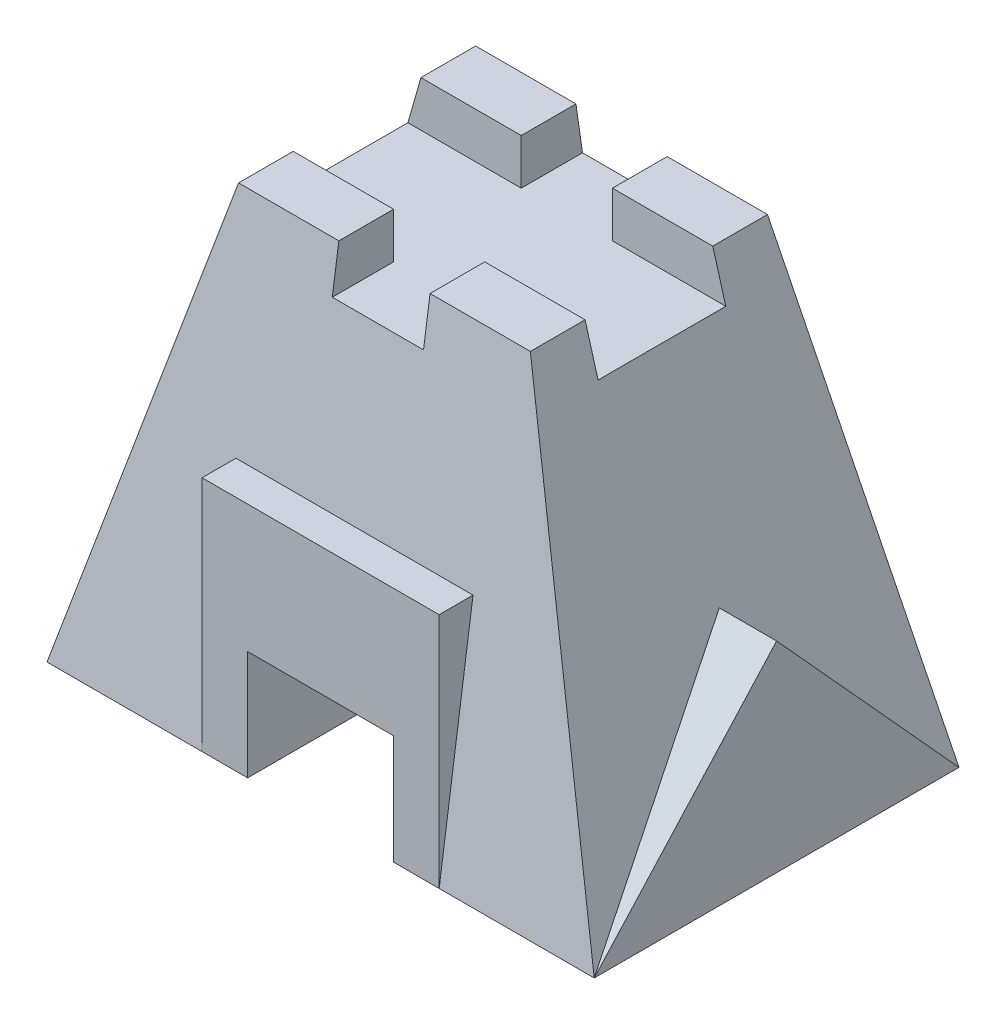
ISO-10303-21;
HEADER;
FILE_DESCRIPTION(('STEP AP214'),'2;1');
FILE_NAME('part.step','',(''),(''),'','','');
FILE_SCHEMA(('AUTOMOTIVE_DESIGN { 1 0 10303 214 1 1 1 1 }'));
ENDSEC;
DATA;
#1=APPLICATION_CONTEXT('core data for automotive mechanical design processes');
#2=APPLICATION_PROTOCOL_DEFINITION('international standard','automotive_design',2000,#1);
#3=PRODUCT_CONTEXT('',#1,'mechanical');
#4=PRODUCT('Part','Part','',(#3));
#5=PRODUCT_RELATED_PRODUCT_CATEGORY('part','',(#4));
#6=PRODUCT_DEFINITION_FORMATION('','',#4);
#7=PRODUCT_DEFINITION_CONTEXT('part definition',#1,'design');
#8=PRODUCT_DEFINITION('design','',#6,#7);
#9=PRODUCT_DEFINITION_SHAPE('','',#8);
#10=(LENGTH_UNIT() NAMED_UNIT(*) SI_UNIT(.MILLI.,.METRE.));
#11=(NAMED_UNIT(*) PLANE_ANGLE_UNIT() SI_UNIT($,.RADIAN.));
#12=(NAMED_UNIT(*) SI_UNIT($,.STERADIAN.) SOLID_ANGLE_UNIT());
#13=UNCERTAINTY_MEASURE_WITH_UNIT(LENGTH_MEASURE(1.E-05),#10,'distance_accuracy_value','');
#14=(GEOMETRIC_REPRESENTATION_CONTEXT(3) GLOBAL_UNCERTAINTY_ASSIGNED_CONTEXT((#13)) GLOBAL_UNIT_ASSIGNED_CONTEXT((#10,
#11,#12)) REPRESENTATION_CONTEXT('',''));
#15=CARTESIAN_POINT('',(0.,0.,0.));
#16=DIRECTION('',(0.,0.,1.));
#17=DIRECTION('',(1.,0.,0.));
#18=AXIS2_PLACEMENT_3D('',#15,#16,#17);
#19=CARTESIAN_POINT('',(0.,245.,0.));
#20=DIRECTION('',(0.,-1.,0.));
#21=DIRECTION('',(0.,0.,-1.));
#22=AXIS2_PLACEMENT_3D('',#19,#20,#21);
#23=PLANE('',#22);
#24=DIRECTION('',(-1.,0.,0.));
#25=VECTOR('',#24,1.);
#26=CARTESIAN_POINT('',(-80.,245.,-65.));
#27=LINE('',#26,#25);
#28=CARTESIAN_POINT('',(80.,245.,-65.));
#29=VERTEX_POINT('',#28);
#30=CARTESIAN_POINT('',(25.,245.,-65.));
#31=VERTEX_POINT('',#30);
#32=EDGE_CURVE('E51',#29,#31,#27,.T.);
#33=ORIENTED_EDGE('',*,*,#32,.T.);
#34=DIRECTION('',(0.,0.,-1.));
#35=VECTOR('',#34,1.);
#36=CARTESIAN_POINT('',(25.,245.,-74.6053871623696));
#37=LINE('',#36,#35);
#38=CARTESIAN_POINT('',(25.,245.,-35.));
#39=VERTEX_POINT('',#38);
#40=EDGE_CURVE('E244',#39,#31,#37,.T.);
#41=ORIENTED_EDGE('',*,*,#40,.F.);
#42=DIRECTION('',(1.,0.,0.));
#43=VECTOR('',#42,1.);
#44=CARTESIAN_POINT('',(0.,245.,-35.));
#45=LINE('',#44,#43);
#46=CARTESIAN_POINT('',(80.,245.,-35.));
#47=VERTEX_POINT('',#46);
#48=EDGE_CURVE('E60',#39,#47,#45,.T.);
#49=ORIENTED_EDGE('',*,*,#48,.T.);
#50=DIRECTION('',(0.,0.,-1.));
#51=VECTOR('',#50,1.);
#52=CARTESIAN_POINT('',(80.,245.,65.));
#53=LINE('',#52,#51);
#54=EDGE_CURVE('E428',#47,#29,#53,.T.);
#55=ORIENTED_EDGE('',*,*,#54,.T.);
#56=EDGE_LOOP('',(#33,#41,#49,#55));
#57=FACE_BOUND('',#56,.T.);
#58=ADVANCED_FACE('F50',(#57),#23,.F.);
#59=CARTESIAN_POINT('',(80.,245.,65.));
#60=VERTEX_POINT('',#59);
#61=CARTESIAN_POINT('',(80.,245.,35.));
#62=VERTEX_POINT('',#61);
#63=EDGE_CURVE('E536',#60,#62,#53,.T.);
#64=ORIENTED_EDGE('',*,*,#63,.T.);
#65=DIRECTION('',(1.,0.,0.));
#66=VECTOR('',#65,1.);
#67=CARTESIAN_POINT('',(80.,245.,35.));
#68=LINE('',#67,#66);
#69=CARTESIAN_POINT('',(25.,245.,35.));
#70=VERTEX_POINT('',#69);
#71=EDGE_CURVE('E292',#70,#62,#68,.T.);
#72=ORIENTED_EDGE('',*,*,#71,.F.);
#73=DIRECTION('',(0.,0.,1.));
#74=VECTOR('',#73,1.);
#75=CARTESIAN_POINT('',(25.,245.,0.));
#76=LINE('',#75,#74);
#77=CARTESIAN_POINT('',(25.,245.,65.));
#78=VERTEX_POINT('',#77);
#79=EDGE_CURVE('E552',#70,#78,#76,.T.);
#80=ORIENTED_EDGE('',*,*,#79,.T.);
#81=DIRECTION('',(1.,0.,0.));
#82=VECTOR('',#81,1.);
#83=CARTESIAN_POINT('',(-80.,245.,65.));
#84=LINE('',#83,#82);
#85=EDGE_CURVE('E531',#78,#60,#84,.T.);
#86=ORIENTED_EDGE('',*,*,#85,.T.);
#87=EDGE_LOOP('',(#64,#72,#80,#86));
#88=FACE_BOUND('',#87,.T.);
#89=ADVANCED_FACE('F750',(#88),#23,.F.);
#90=CARTESIAN_POINT('',(-80.,245.,65.));
#91=VERTEX_POINT('',#90);
#92=CARTESIAN_POINT('',(-25.,245.,65.));
#93=VERTEX_POINT('',#92);
#94=EDGE_CURVE('E529',#91,#93,#84,.T.);
#95=ORIENTED_EDGE('',*,*,#94,.T.);
#96=DIRECTION('',(0.,0.,1.));
#97=VECTOR('',#96,1.);
#98=CARTESIAN_POINT('',(-25.,245.,65.));
#99=LINE('',#98,#97);
#100=CARTESIAN_POINT('',(-25.,245.,35.));
#101=VERTEX_POINT('',#100);
#102=EDGE_CURVE('E276',#101,#93,#99,.T.);
#103=ORIENTED_EDGE('',*,*,#102,.F.);
#104=DIRECTION('',(-1.,0.,0.));
#105=VECTOR('',#104,1.);
#106=CARTESIAN_POINT('',(0.,245.,35.));
#107=LINE('',#106,#105);
#108=CARTESIAN_POINT('',(-80.,245.,35.));
#109=VERTEX_POINT('',#108);
#110=EDGE_CURVE('E557',#101,#109,#107,.T.);
#111=ORIENTED_EDGE('',*,*,#110,.T.);
#112=DIRECTION('',(0.,0.,1.));
#113=VECTOR('',#112,1.);
#114=CARTESIAN_POINT('',(-80.,245.,65.));
#115=LINE('',#114,#113);
#116=EDGE_CURVE('E545',#109,#91,#115,.T.);
#117=ORIENTED_EDGE('',*,*,#116,.T.);
#118=EDGE_LOOP('',(#95,#103,#111,#117));
#119=FACE_BOUND('',#118,.T.);
#120=ADVANCED_FACE('F451',(#119),#23,.F.);
#121=CARTESIAN_POINT('',(0.,0.,0.));
#122=DIRECTION('',(0.,-1.,0.));
#123=DIRECTION('',(0.,0.,-1.));
#124=AXIS2_PLACEMENT_3D('',#121,#122,#123);
#125=PLANE('',#124);
#126=DIRECTION('',(0.,0.,1.));
#127=VECTOR('',#126,1.);
#128=CARTESIAN_POINT('',(-40.,0.,-100.0001));
#129=LINE('',#128,#127);
#130=CARTESIAN_POINT('',(-40.,0.,-100.));
#131=VERTEX_POINT('',#130);
#132=CARTESIAN_POINT('',(-40.,0.,100.));
#133=VERTEX_POINT('',#132);
#134=EDGE_CURVE('E322',#131,#133,#129,.T.);
#135=ORIENTED_EDGE('',*,*,#134,.T.);
#136=DIRECTION('',(1.,0.,0.));
#137=VECTOR('',#136,1.);
#138=CARTESIAN_POINT('',(-65.,0.,100.));
#139=LINE('',#138,#137);
#140=CARTESIAN_POINT('',(-65.,0.,100.));
#141=VERTEX_POINT('',#140);
#142=EDGE_CURVE('E411',#141,#133,#139,.T.);
#143=ORIENTED_EDGE('',*,*,#142,.F.);
#144=DIRECTION('',(1.,0.,0.));
#145=VECTOR('',#144,1.);
#146=CARTESIAN_POINT('',(-150.,0.,100.));
#147=LINE('',#146,#145);
#148=CARTESIAN_POINT('',(-150.,0.,100.));
#149=VERTEX_POINT('',#148);
#150=EDGE_CURVE('E665',#149,#141,#147,.T.);
#151=ORIENTED_EDGE('',*,*,#150,.F.);
#152=DIRECTION('',(0.,0.,1.));
#153=VECTOR('',#152,1.);
#154=CARTESIAN_POINT('',(-150.,0.,100.));
#155=LINE('',#154,#153);
#156=CARTESIAN_POINT('',(-150.,0.,-100.));
#157=VERTEX_POINT('',#156);
#158=EDGE_CURVE('E654',#157,#149,#155,.T.);
#159=ORIENTED_EDGE('',*,*,#158,.F.);
#160=DIRECTION('',(-1.,0.,0.));
#161=VECTOR('',#160,1.);
#162=CARTESIAN_POINT('',(-150.,0.,-100.));
#163=LINE('',#162,#161);
#164=CARTESIAN_POINT('',(-65.,0.,-100.));
#165=VERTEX_POINT('',#164);
#166=EDGE_CURVE('E650',#165,#157,#163,.T.);
#167=ORIENTED_EDGE('',*,*,#166,.F.);
#168=DIRECTION('',(1.,0.,0.));
#169=VECTOR('',#168,1.);
#170=CARTESIAN_POINT('',(-65.,0.,-100.));
#171=LINE('',#170,#169);
#172=EDGE_CURVE('E406',#165,#131,#171,.T.);
#173=ORIENTED_EDGE('',*,*,#172,.T.);
#174=EDGE_LOOP('',(#135,#143,#151,#159,#167,#173));
#175=FACE_BOUND('',#174,.T.);
#176=ADVANCED_FACE('F709',(#175),#125,.T.);
#177=CARTESIAN_POINT('',(-138.679245283019,39.622641509434,0.));
#178=DIRECTION('',(-0.961523947640823,0.274721127897378,0.));
#179=DIRECTION('',(-0.274721127897378,-0.961523947640823,0.));
#180=AXIS2_PLACEMENT_3D('',#177,#178,#179);
#181=PLANE('',#180);
#182=DIRECTION('',(0.274721127897378,0.961523947640823,0.));
#183=VECTOR('',#182,1.);
#184=CARTESIAN_POINT('',(-138.679245283019,39.622641509434,35.));
#185=LINE('',#184,#183);
#186=CARTESIAN_POINT('',(-87.1428571428572,220.,35.));
#187=VERTEX_POINT('',#186);
#188=EDGE_CURVE('E285',#187,#109,#185,.T.);
#189=ORIENTED_EDGE('',*,*,#188,.F.);
#190=DIRECTION('',(0.,0.,1.));
#191=VECTOR('',#190,1.);
#192=CARTESIAN_POINT('',(-87.1428571428572,220.,0.));
#193=LINE('',#192,#191);
#194=CARTESIAN_POINT('',(-87.1428571428572,220.,-35.));
#195=VERTEX_POINT('',#194);
#196=EDGE_CURVE('E325',#195,#187,#193,.T.);
#197=ORIENTED_EDGE('',*,*,#196,.F.);
#198=DIRECTION('',(-0.274721127897378,-0.961523947640823,0.));
#199=VECTOR('',#198,1.);
#200=CARTESIAN_POINT('',(-138.679245283019,39.622641509434,-35.));
#201=LINE('',#200,#199);
#202=CARTESIAN_POINT('',(-80.,245.,-35.));
#203=VERTEX_POINT('',#202);
#204=EDGE_CURVE('E254',#203,#195,#201,.T.);
#205=ORIENTED_EDGE('',*,*,#204,.F.);
#206=CARTESIAN_POINT('',(-80.,245.,-65.));
#207=VERTEX_POINT('',#206);
#208=EDGE_CURVE('E532',#207,#203,#115,.T.);
#209=ORIENTED_EDGE('',*,*,#208,.F.);
#210=DIRECTION('',(-0.272165526975909,-0.95257934441568,-0.136082763487954));
#211=VECTOR('',#210,1.);
#212=CARTESIAN_POINT('',(-80.,245.,-65.));
#213=LINE('',#212,#211);
#214=EDGE_CURVE('E581',#207,#157,#213,.T.);
#215=ORIENTED_EDGE('',*,*,#214,.T.);
#216=DIRECTION('',(0.20683964668639,0.723938763402365,0.658126148547605));
#217=VECTOR('',#216,1.);
#218=CARTESIAN_POINT('',(-129.969946079731,70.1051887209405,-36.2680102536904));
#219=LINE('',#218,#217);
#220=CARTESIAN_POINT('',(-118.571428571429,110.,0.));
#221=VERTEX_POINT('',#220);
#222=EDGE_CURVE('E367',#157,#221,#219,.T.);
#223=ORIENTED_EDGE('',*,*,#222,.T.);
#224=DIRECTION('',(-0.20683964668639,-0.723938763402365,0.658126148547605));
#225=VECTOR('',#224,1.);
#226=CARTESIAN_POINT('',(-129.969946079731,70.1051887209405,36.2680102536904));
#227=LINE('',#226,#225);
#228=EDGE_CURVE('E355',#221,#149,#227,.T.);
#229=ORIENTED_EDGE('',*,*,#228,.T.);
#230=DIRECTION('',(-0.272165526975909,-0.95257934441568,0.136082763487954));
#231=VECTOR('',#230,1.);
#232=CARTESIAN_POINT('',(-80.,245.,65.));
#233=LINE('',#232,#231);
#234=EDGE_CURVE('E573',#91,#149,#233,.T.);
#235=ORIENTED_EDGE('',*,*,#234,.F.);
#236=ORIENTED_EDGE('',*,*,#116,.F.);
#237=EDGE_LOOP('',(#189,#197,#205,#209,#215,#223,#229,#235,#236));
#238=FACE_BOUND('',#237,.T.);
#239=ADVANCED_FACE('F460',(#238),#181,.T.);
#240=CARTESIAN_POINT('',(138.679245283019,39.6226415094339,0.));
#241=DIRECTION('',(0.961523947640823,0.274721127897378,0.));
#242=DIRECTION('',(-0.274721127897378,0.961523947640823,0.));
#243=AXIS2_PLACEMENT_3D('',#240,#241,#242);
#244=PLANE('',#243);
#245=DIRECTION('',(-0.274721127897378,0.961523947640823,0.));
#246=VECTOR('',#245,1.);
#247=CARTESIAN_POINT('',(138.679245283019,39.6226415094339,-35.));
#248=LINE('',#247,#246);
#249=CARTESIAN_POINT('',(87.1428571428571,220.,-35.));
#250=VERTEX_POINT('',#249);
#251=EDGE_CURVE('E316',#250,#47,#248,.T.);
#252=ORIENTED_EDGE('',*,*,#251,.F.);
#253=DIRECTION('',(0.,0.,-1.));
#254=VECTOR('',#253,1.);
#255=CARTESIAN_POINT('',(87.1428571428571,220.,0.));
#256=LINE('',#255,#254);
#257=CARTESIAN_POINT('',(87.1428571428571,220.,35.));
#258=VERTEX_POINT('',#257);
#259=EDGE_CURVE('E319',#258,#250,#256,.T.);
#260=ORIENTED_EDGE('',*,*,#259,.F.);
#261=DIRECTION('',(0.274721127897378,-0.961523947640823,0.));
#262=VECTOR('',#261,1.);
#263=CARTESIAN_POINT('',(138.679245283019,39.6226415094339,35.));
#264=LINE('',#263,#262);
#265=EDGE_CURVE('E299',#62,#258,#264,.T.);
#266=ORIENTED_EDGE('',*,*,#265,.F.);
#267=ORIENTED_EDGE('',*,*,#63,.F.);
#268=DIRECTION('',(0.272165526975909,-0.95257934441568,0.136082763487954));
#269=VECTOR('',#268,1.);
#270=CARTESIAN_POINT('',(80.,245.,65.));
#271=LINE('',#270,#269);
#272=CARTESIAN_POINT('',(150.,0.,100.));
#273=VERTEX_POINT('',#272);
#274=EDGE_CURVE('E588',#60,#273,#271,.T.);
#275=ORIENTED_EDGE('',*,*,#274,.T.);
#276=DIRECTION('',(-0.20683964668639,0.723938763402365,-0.658126148547605));
#277=VECTOR('',#276,1.);
#278=CARTESIAN_POINT('',(129.969946079731,70.1051887209405,36.2680102536904));
#279=LINE('',#278,#277);
#280=CARTESIAN_POINT('',(118.571428571429,110.,0.));
#281=VERTEX_POINT('',#280);
#282=EDGE_CURVE('E341',#273,#281,#279,.T.);
#283=ORIENTED_EDGE('',*,*,#282,.T.);
#284=DIRECTION('',(0.20683964668639,-0.723938763402365,-0.658126148547605));
#285=VECTOR('',#284,1.);
#286=CARTESIAN_POINT('',(129.969946079731,70.1051887209405,-36.2680102536904));
#287=LINE('',#286,#285);
#288=CARTESIAN_POINT('',(150.,0.,-100.));
#289=VERTEX_POINT('',#288);
#290=EDGE_CURVE('E365',#281,#289,#287,.T.);
#291=ORIENTED_EDGE('',*,*,#290,.T.);
#292=DIRECTION('',(0.272165526975909,-0.95257934441568,-0.136082763487954));
#293=VECTOR('',#292,1.);
#294=CARTESIAN_POINT('',(80.,245.,-65.));
#295=LINE('',#294,#293);
#296=EDGE_CURVE('E500',#29,#289,#295,.T.);
#297=ORIENTED_EDGE('',*,*,#296,.F.);
#298=ORIENTED_EDGE('',*,*,#54,.F.);
#299=EDGE_LOOP('',(#252,#260,#266,#267,#275,#283,#291,#297,#298));
#300=FACE_BOUND('',#299,.T.);
#301=ADVANCED_FACE('F508',(#300),#244,.T.);
#302=CARTESIAN_POINT('',(0.,14.,98.));
#303=DIRECTION('',(0.,0.141421356237309,0.989949493661167));
#304=DIRECTION('',(0.,-0.989949493661167,0.141421356237309));
#305=AXIS2_PLACEMENT_3D('',#302,#303,#304);
#306=PLANE('',#305);
#307=DIRECTION('',(0.,0.989949493661167,-0.141421356237309));
#308=VECTOR('',#307,1.);
#309=CARTESIAN_POINT('',(25.0000000000001,14.,98.));
#310=LINE('',#309,#308);
#311=CARTESIAN_POINT('',(25.,220.,68.5714285714286));
#312=VERTEX_POINT('',#311);
#313=EDGE_CURVE('E291',#312,#78,#310,.T.);
#314=ORIENTED_EDGE('',*,*,#313,.F.);
#315=DIRECTION('',(1.,0.,0.));
#316=VECTOR('',#315,1.);
#317=CARTESIAN_POINT('',(0.,220.,68.5714285714286));
#318=LINE('',#317,#316);
#319=CARTESIAN_POINT('',(-25.,220.,68.5714285714286));
#320=VERTEX_POINT('',#319);
#321=EDGE_CURVE('E312',#320,#312,#318,.T.);
#322=ORIENTED_EDGE('',*,*,#321,.F.);
#323=DIRECTION('',(0.,-0.989949493661167,0.141421356237309));
#324=VECTOR('',#323,1.);
#325=CARTESIAN_POINT('',(-25.,14.,98.));
#326=LINE('',#325,#324);
#327=EDGE_CURVE('E290',#93,#320,#326,.T.);
#328=ORIENTED_EDGE('',*,*,#327,.F.);
#329=ORIENTED_EDGE('',*,*,#94,.F.);
#330=ORIENTED_EDGE('',*,*,#234,.T.);
#331=ORIENTED_EDGE('',*,*,#150,.T.);
#332=DIRECTION('',(0.,0.989949493661167,-0.141421356237309));
#333=VECTOR('',#332,1.);
#334=CARTESIAN_POINT('',(-65.,14.,98.));
#335=LINE('',#334,#333);
#336=CARTESIAN_POINT('',(-65.,130.,81.4285714285714));
#337=VERTEX_POINT('',#336);
#338=EDGE_CURVE('E393',#141,#337,#335,.T.);
#339=ORIENTED_EDGE('',*,*,#338,.T.);
#340=DIRECTION('',(1.,0.,0.));
#341=VECTOR('',#340,1.);
#342=CARTESIAN_POINT('',(0.,130.,81.4285714285714));
#343=LINE('',#342,#341);
#344=CARTESIAN_POINT('',(65.,130.,81.4285714285714));
#345=VERTEX_POINT('',#344);
#346=EDGE_CURVE('E399',#337,#345,#343,.T.);
#347=ORIENTED_EDGE('',*,*,#346,.T.);
#348=DIRECTION('',(0.,-0.989949493661167,0.141421356237309));
#349=VECTOR('',#348,1.);
#350=CARTESIAN_POINT('',(65.,14.,98.));
#351=LINE('',#350,#349);
#352=CARTESIAN_POINT('',(65.,0.,100.));
#353=VERTEX_POINT('',#352);
#354=EDGE_CURVE('E688',#345,#353,#351,.T.);
#355=ORIENTED_EDGE('',*,*,#354,.T.);
#356=EDGE_CURVE('E657',#353,#273,#147,.T.);
#357=ORIENTED_EDGE('',*,*,#356,.T.);
#358=ORIENTED_EDGE('',*,*,#274,.F.);
#359=ORIENTED_EDGE('',*,*,#85,.F.);
#360=EDGE_LOOP('',(#314,#322,#328,#329,#330,#331,#339,#347,#355,#357,#358,#359));
#361=FACE_BOUND('',#360,.T.);
#362=ADVANCED_FACE('F509',(#361),#306,.T.);
#363=CARTESIAN_POINT('',(0.,14.,-98.));
#364=DIRECTION('',(0.,0.14142135623731,-0.989949493661167));
#365=DIRECTION('',(0.,0.989949493661167,0.14142135623731));
#366=AXIS2_PLACEMENT_3D('',#363,#364,#365);
#367=PLANE('',#366);
#368=DIRECTION('',(0.,-0.989949493661167,-0.14142135623731));
#369=VECTOR('',#368,1.);
#370=CARTESIAN_POINT('',(25.,14.,-98.));
#371=LINE('',#370,#369);
#372=CARTESIAN_POINT('',(25.,220.,-68.5714285714286));
#373=VERTEX_POINT('',#372);
#374=EDGE_CURVE('E311',#31,#373,#371,.T.);
#375=ORIENTED_EDGE('',*,*,#374,.F.);
#376=ORIENTED_EDGE('',*,*,#32,.F.);
#377=ORIENTED_EDGE('',*,*,#296,.T.);
#378=CARTESIAN_POINT('',(65.,0.,-100.));
#379=VERTEX_POINT('',#378);
#380=EDGE_CURVE('E647',#289,#379,#163,.T.);
#381=ORIENTED_EDGE('',*,*,#380,.T.);
#382=DIRECTION('',(0.,0.989949493661167,0.14142135623731));
#383=VECTOR('',#382,1.);
#384=CARTESIAN_POINT('',(65.,14.,-98.));
#385=LINE('',#384,#383);
#386=CARTESIAN_POINT('',(65.,130.,-81.4285714285714));
#387=VERTEX_POINT('',#386);
#388=EDGE_CURVE('E677',#379,#387,#385,.T.);
#389=ORIENTED_EDGE('',*,*,#388,.T.);
#390=DIRECTION('',(-1.,0.,0.));
#391=VECTOR('',#390,1.);
#392=CARTESIAN_POINT('',(0.,130.,-81.4285714285714));
#393=LINE('',#392,#391);
#394=CARTESIAN_POINT('',(-65.,130.,-81.4285714285714));
#395=VERTEX_POINT('',#394);
#396=EDGE_CURVE('E675',#387,#395,#393,.T.);
#397=ORIENTED_EDGE('',*,*,#396,.T.);
#398=DIRECTION('',(0.,-0.989949493661167,-0.14142135623731));
#399=VECTOR('',#398,1.);
#400=CARTESIAN_POINT('',(-65.,14.,-98.));
#401=LINE('',#400,#399);
#402=EDGE_CURVE('E661',#395,#165,#401,.T.);
#403=ORIENTED_EDGE('',*,*,#402,.T.);
#404=ORIENTED_EDGE('',*,*,#166,.T.);
#405=ORIENTED_EDGE('',*,*,#214,.F.);
#406=CARTESIAN_POINT('',(-25.0000000000001,245.,-65.));
#407=VERTEX_POINT('',#406);
#408=EDGE_CURVE('E482',#407,#207,#27,.T.);
#409=ORIENTED_EDGE('',*,*,#408,.F.);
#410=DIRECTION('',(0.,0.989949493661167,0.14142135623731));
#411=VECTOR('',#410,1.);
#412=CARTESIAN_POINT('',(-25.0000000000001,14.,-98.));
#413=LINE('',#412,#411);
#414=CARTESIAN_POINT('',(-25.,220.,-68.5714285714286));
#415=VERTEX_POINT('',#414);
#416=EDGE_CURVE('E63',#415,#407,#413,.T.);
#417=ORIENTED_EDGE('',*,*,#416,.F.);
#418=DIRECTION('',(-1.,0.,0.));
#419=VECTOR('',#418,1.);
#420=CARTESIAN_POINT('',(0.,220.,-68.5714285714286));
#421=LINE('',#420,#419);
#422=EDGE_CURVE('E12',#373,#415,#421,.T.);
#423=ORIENTED_EDGE('',*,*,#422,.F.);
#424=EDGE_LOOP('',(#375,#376,#377,#381,#389,#397,#403,#404,#405,#409,#417,#423));
#425=FACE_BOUND('',#424,.T.);
#426=ADVANCED_FACE('F498',(#425),#367,.T.);
#427=DIRECTION('',(0.,0.,1.));
#428=VECTOR('',#427,1.);
#429=CARTESIAN_POINT('',(40.,0.,-100.0001));
#430=LINE('',#429,#428);
#431=CARTESIAN_POINT('',(40.,0.,-100.));
#432=VERTEX_POINT('',#431);
#433=CARTESIAN_POINT('',(40.,0.,100.));
#434=VERTEX_POINT('',#433);
#435=EDGE_CURVE('E71',#432,#434,#430,.T.);
#436=ORIENTED_EDGE('',*,*,#435,.F.);
#437=EDGE_CURVE('E373',#432,#379,#171,.T.);
#438=ORIENTED_EDGE('',*,*,#437,.T.);
#439=ORIENTED_EDGE('',*,*,#380,.F.);
#440=DIRECTION('',(0.,0.,-1.));
#441=VECTOR('',#440,1.);
#442=CARTESIAN_POINT('',(150.,0.,100.));
#443=LINE('',#442,#441);
#444=EDGE_CURVE('E589',#273,#289,#443,.T.);
#445=ORIENTED_EDGE('',*,*,#444,.F.);
#446=ORIENTED_EDGE('',*,*,#356,.F.);
#447=EDGE_CURVE('E685',#434,#353,#139,.T.);
#448=ORIENTED_EDGE('',*,*,#447,.F.);
#449=EDGE_LOOP('',(#436,#438,#439,#445,#446,#448));
#450=FACE_BOUND('',#449,.T.);
#451=ADVANCED_FACE('F47',(#450),#125,.T.);
#452=ORIENTED_EDGE('',*,*,#208,.T.);
#453=DIRECTION('',(-1.,0.,0.));
#454=VECTOR('',#453,1.);
#455=CARTESIAN_POINT('',(-80.,245.,-35.));
#456=LINE('',#455,#454);
#457=CARTESIAN_POINT('',(-25.,245.,-35.));
#458=VERTEX_POINT('',#457);
#459=EDGE_CURVE('E277',#458,#203,#456,.T.);
#460=ORIENTED_EDGE('',*,*,#459,.F.);
#461=DIRECTION('',(0.,0.,-1.));
#462=VECTOR('',#461,1.);
#463=CARTESIAN_POINT('',(-25.,245.,0.));
#464=LINE('',#463,#462);
#465=EDGE_CURVE('E250',#458,#407,#464,.T.);
#466=ORIENTED_EDGE('',*,*,#465,.T.);
#467=ORIENTED_EDGE('',*,*,#408,.T.);
#468=EDGE_LOOP('',(#452,#460,#466,#467));
#469=FACE_BOUND('',#468,.T.);
#470=ADVANCED_FACE('F445',(#469),#23,.F.);
#471=CARTESIAN_POINT('',(0.,0.,-100.));
#472=DIRECTION('',(0.,0.,-1.));
#473=DIRECTION('',(-1.,0.,0.));
#474=AXIS2_PLACEMENT_3D('',#471,#472,#473);
#475=PLANE('',#474);
#476=DIRECTION('',(0.,1.,0.));
#477=VECTOR('',#476,1.);
#478=CARTESIAN_POINT('',(-40.,0.,-100.));
#479=LINE('',#478,#477);
#480=CARTESIAN_POINT('',(-40.,60.,-100.));
#481=VERTEX_POINT('',#480);
#482=EDGE_CURVE('E340',#131,#481,#479,.T.);
#483=ORIENTED_EDGE('',*,*,#482,.F.);
#484=ORIENTED_EDGE('',*,*,#172,.F.);
#485=DIRECTION('',(0.,-1.,0.));
#486=VECTOR('',#485,1.);
#487=CARTESIAN_POINT('',(-65.,0.,-100.));
#488=LINE('',#487,#486);
#489=CARTESIAN_POINT('',(-65.,130.,-100.));
#490=VERTEX_POINT('',#489);
#491=EDGE_CURVE('E384',#490,#165,#488,.T.);
#492=ORIENTED_EDGE('',*,*,#491,.F.);
#493=DIRECTION('',(-1.,0.,0.));
#494=VECTOR('',#493,1.);
#495=CARTESIAN_POINT('',(-65.,130.,-100.));
#496=LINE('',#495,#494);
#497=CARTESIAN_POINT('',(65.,130.,-100.));
#498=VERTEX_POINT('',#497);
#499=EDGE_CURVE('E385',#498,#490,#496,.T.);
#500=ORIENTED_EDGE('',*,*,#499,.F.);
#501=DIRECTION('',(0.,1.,0.));
#502=VECTOR('',#501,1.);
#503=CARTESIAN_POINT('',(65.,130.,-100.));
#504=LINE('',#503,#502);
#505=EDGE_CURVE('E387',#379,#498,#504,.T.);
#506=ORIENTED_EDGE('',*,*,#505,.F.);
#507=ORIENTED_EDGE('',*,*,#437,.F.);
#508=DIRECTION('',(0.,-1.,0.));
#509=VECTOR('',#508,1.);
#510=CARTESIAN_POINT('',(40.,0.,-100.));
#511=LINE('',#510,#509);
#512=CARTESIAN_POINT('',(40.,60.,-100.));
#513=VERTEX_POINT('',#512);
#514=EDGE_CURVE('E327',#513,#432,#511,.T.);
#515=ORIENTED_EDGE('',*,*,#514,.F.);
#516=DIRECTION('',(1.,0.,0.));
#517=VECTOR('',#516,1.);
#518=CARTESIAN_POINT('',(0.,60.,-100.));
#519=LINE('',#518,#517);
#520=EDGE_CURVE('E337',#481,#513,#519,.T.);
#521=ORIENTED_EDGE('',*,*,#520,.F.);
#522=EDGE_LOOP('',(#483,#484,#492,#500,#506,#507,#515,#521));
#523=FACE_BOUND('',#522,.T.);
#524=ADVANCED_FACE('F455',(#523),#475,.T.);
#525=CARTESIAN_POINT('',(-65.,0.,100.));
#526=DIRECTION('',(1.,0.,0.));
#527=DIRECTION('',(0.,0.,-1.));
#528=AXIS2_PLACEMENT_3D('',#525,#526,#527);
#529=PLANE('',#528);
#530=ORIENTED_EDGE('',*,*,#402,.F.);
#531=DIRECTION('',(0.,0.,-1.));
#532=VECTOR('',#531,1.);
#533=CARTESIAN_POINT('',(-65.,130.,100.));
#534=LINE('',#533,#532);
#535=EDGE_CURVE('E392',#395,#490,#534,.T.);
#536=ORIENTED_EDGE('',*,*,#535,.T.);
#537=ORIENTED_EDGE('',*,*,#491,.T.);
#538=EDGE_LOOP('',(#530,#536,#537));
#539=FACE_BOUND('',#538,.T.);
#540=ADVANCED_FACE('F734',(#539),#529,.F.);
#541=CARTESIAN_POINT('',(-65.,130.,100.));
#542=DIRECTION('',(0.,-1.,0.));
#543=DIRECTION('',(0.,0.,-1.));
#544=AXIS2_PLACEMENT_3D('',#541,#542,#543);
#545=PLANE('',#544);
#546=ORIENTED_EDGE('',*,*,#396,.F.);
#547=DIRECTION('',(0.,0.,-1.));
#548=VECTOR('',#547,1.);
#549=CARTESIAN_POINT('',(65.,130.,100.));
#550=LINE('',#549,#548);
#551=EDGE_CURVE('E388',#387,#498,#550,.T.);
#552=ORIENTED_EDGE('',*,*,#551,.T.);
#553=ORIENTED_EDGE('',*,*,#499,.T.);
#554=ORIENTED_EDGE('',*,*,#535,.F.);
#555=EDGE_LOOP('',(#546,#552,#553,#554));
#556=FACE_BOUND('',#555,.T.);
#557=ADVANCED_FACE('F728',(#556),#545,.F.);
#558=CARTESIAN_POINT('',(65.,130.,100.));
#559=DIRECTION('',(-1.,0.,0.));
#560=DIRECTION('',(0.,0.,1.));
#561=AXIS2_PLACEMENT_3D('',#558,#559,#560);
#562=PLANE('',#561);
#563=ORIENTED_EDGE('',*,*,#388,.F.);
#564=ORIENTED_EDGE('',*,*,#505,.T.);
#565=ORIENTED_EDGE('',*,*,#551,.F.);
#566=EDGE_LOOP('',(#563,#564,#565));
#567=FACE_BOUND('',#566,.T.);
#568=ADVANCED_FACE('F453',(#567),#562,.F.);
#569=ORIENTED_EDGE('',*,*,#354,.F.);
#570=CARTESIAN_POINT('',(65.,130.,100.));
#571=VERTEX_POINT('',#570);
#572=EDGE_CURVE('E394',#571,#345,#550,.T.);
#573=ORIENTED_EDGE('',*,*,#572,.F.);
#574=DIRECTION('',(0.,1.,0.));
#575=VECTOR('',#574,1.);
#576=CARTESIAN_POINT('',(65.,130.,100.));
#577=LINE('',#576,#575);
#578=EDGE_CURVE('E381',#353,#571,#577,.T.);
#579=ORIENTED_EDGE('',*,*,#578,.F.);
#580=EDGE_LOOP('',(#569,#573,#579));
#581=FACE_BOUND('',#580,.T.);
#582=ADVANCED_FACE('F762',(#581),#562,.F.);
#583=ORIENTED_EDGE('',*,*,#346,.F.);
#584=CARTESIAN_POINT('',(-65.,130.,100.));
#585=VERTEX_POINT('',#584);
#586=EDGE_CURVE('E390',#585,#337,#534,.T.);
#587=ORIENTED_EDGE('',*,*,#586,.F.);
#588=DIRECTION('',(-1.,0.,0.));
#589=VECTOR('',#588,1.);
#590=CARTESIAN_POINT('',(-65.,130.,100.));
#591=LINE('',#590,#589);
#592=EDGE_CURVE('E378',#571,#585,#591,.T.);
#593=ORIENTED_EDGE('',*,*,#592,.F.);
#594=ORIENTED_EDGE('',*,*,#572,.T.);
#595=EDGE_LOOP('',(#583,#587,#593,#594));
#596=FACE_BOUND('',#595,.T.);
#597=ADVANCED_FACE('F744',(#596),#545,.F.);
#598=ORIENTED_EDGE('',*,*,#338,.F.);
#599=DIRECTION('',(0.,-1.,0.));
#600=VECTOR('',#599,1.);
#601=CARTESIAN_POINT('',(-65.,0.,100.));
#602=LINE('',#601,#600);
#603=EDGE_CURVE('E379',#585,#141,#602,.T.);
#604=ORIENTED_EDGE('',*,*,#603,.F.);
#605=ORIENTED_EDGE('',*,*,#586,.T.);
#606=EDGE_LOOP('',(#598,#604,#605));
#607=FACE_BOUND('',#606,.T.);
#608=ADVANCED_FACE('F739',(#607),#529,.F.);
#609=CARTESIAN_POINT('',(0.,0.,100.));
#610=DIRECTION('',(0.,0.,-1.));
#611=DIRECTION('',(-1.,0.,0.));
#612=AXIS2_PLACEMENT_3D('',#609,#610,#611);
#613=PLANE('',#612);
#614=ORIENTED_EDGE('',*,*,#142,.T.);
#615=DIRECTION('',(0.,1.,0.));
#616=VECTOR('',#615,1.);
#617=CARTESIAN_POINT('',(-40.,0.,100.));
#618=LINE('',#617,#616);
#619=CARTESIAN_POINT('',(-40.,60.,100.));
#620=VERTEX_POINT('',#619);
#621=EDGE_CURVE('E419',#133,#620,#618,.T.);
#622=ORIENTED_EDGE('',*,*,#621,.T.);
#623=DIRECTION('',(1.,0.,0.));
#624=VECTOR('',#623,1.);
#625=CARTESIAN_POINT('',(0.,60.,100.));
#626=LINE('',#625,#624);
#627=CARTESIAN_POINT('',(40.,60.,100.));
#628=VERTEX_POINT('',#627);
#629=EDGE_CURVE('E705',#620,#628,#626,.T.);
#630=ORIENTED_EDGE('',*,*,#629,.T.);
#631=DIRECTION('',(0.,-1.,0.));
#632=VECTOR('',#631,1.);
#633=CARTESIAN_POINT('',(40.,0.,100.));
#634=LINE('',#633,#632);
#635=EDGE_CURVE('E676',#628,#434,#634,.T.);
#636=ORIENTED_EDGE('',*,*,#635,.T.);
#637=ORIENTED_EDGE('',*,*,#447,.T.);
#638=ORIENTED_EDGE('',*,*,#578,.T.);
#639=ORIENTED_EDGE('',*,*,#592,.T.);
#640=ORIENTED_EDGE('',*,*,#603,.T.);
#641=EDGE_LOOP('',(#614,#622,#630,#636,#637,#638,#639,#640));
#642=FACE_BOUND('',#641,.T.);
#643=ADVANCED_FACE('F702',(#642),#613,.F.);
#644=CARTESIAN_POINT('',(150.,0.,0.));
#645=DIRECTION('',(-1.,0.,0.));
#646=DIRECTION('',(0.,0.,1.));
#647=AXIS2_PLACEMENT_3D('',#644,#645,#646);
#648=PLANE('',#647);
#649=ORIENTED_EDGE('',*,*,#444,.T.);
#650=DIRECTION('',(0.,0.739940073395944,0.672672793996313));
#651=VECTOR('',#650,1.);
#652=CARTESIAN_POINT('',(150.,110.,0.));
#653=LINE('',#652,#651);
#654=CARTESIAN_POINT('',(150.,110.,0.));
#655=VERTEX_POINT('',#654);
#656=EDGE_CURVE('E356',#289,#655,#653,.T.);
#657=ORIENTED_EDGE('',*,*,#656,.T.);
#658=DIRECTION('',(0.,-0.739940073395944,0.672672793996313));
#659=VECTOR('',#658,1.);
#660=CARTESIAN_POINT('',(150.,0.,100.));
#661=LINE('',#660,#659);
#662=EDGE_CURVE('E357',#655,#273,#661,.T.);
#663=ORIENTED_EDGE('',*,*,#662,.T.);
#664=EDGE_LOOP('',(#649,#657,#663));
#665=FACE_BOUND('',#664,.T.);
#666=ADVANCED_FACE('F644',(#665),#648,.F.);
#667=CARTESIAN_POINT('',(150.,0.,100.));
#668=DIRECTION('',(0.,-0.672672793996313,-0.739940073395944));
#669=DIRECTION('',(0.,0.739940073395944,-0.672672793996313));
#670=AXIS2_PLACEMENT_3D('',#667,#668,#669);
#671=PLANE('',#670);
#672=ORIENTED_EDGE('',*,*,#282,.F.);
#673=ORIENTED_EDGE('',*,*,#662,.F.);
#674=DIRECTION('',(-1.,0.,0.));
#675=VECTOR('',#674,1.);
#676=CARTESIAN_POINT('',(150.,110.,0.));
#677=LINE('',#676,#675);
#678=EDGE_CURVE('E342',#655,#281,#677,.T.);
#679=ORIENTED_EDGE('',*,*,#678,.T.);
#680=EDGE_LOOP('',(#672,#673,#679));
#681=FACE_BOUND('',#680,.T.);
#682=ADVANCED_FACE('F789',(#681),#671,.F.);
#683=CARTESIAN_POINT('',(150.,110.,0.));
#684=DIRECTION('',(0.,-0.672672793996313,0.739940073395944));
#685=DIRECTION('',(0.,-0.739940073395944,-0.672672793996313));
#686=AXIS2_PLACEMENT_3D('',#683,#684,#685);
#687=PLANE('',#686);
#688=ORIENTED_EDGE('',*,*,#290,.F.);
#689=ORIENTED_EDGE('',*,*,#678,.F.);
#690=ORIENTED_EDGE('',*,*,#656,.F.);
#691=EDGE_LOOP('',(#688,#689,#690));
#692=FACE_BOUND('',#691,.T.);
#693=ADVANCED_FACE('F639',(#692),#687,.F.);
#694=ORIENTED_EDGE('',*,*,#222,.F.);
#695=DIRECTION('',(0.,0.739940073395944,0.672672793996313));
#696=VECTOR('',#695,1.);
#697=CARTESIAN_POINT('',(-150.,110.,0.));
#698=LINE('',#697,#696);
#699=CARTESIAN_POINT('',(-150.,110.,0.));
#700=VERTEX_POINT('',#699);
#701=EDGE_CURVE('E338',#157,#700,#698,.T.);
#702=ORIENTED_EDGE('',*,*,#701,.T.);
#703=EDGE_CURVE('E343',#221,#700,#677,.T.);
#704=ORIENTED_EDGE('',*,*,#703,.F.);
#705=EDGE_LOOP('',(#694,#702,#704));
#706=FACE_BOUND('',#705,.T.);
#707=ADVANCED_FACE('F782',(#706),#687,.F.);
#708=ORIENTED_EDGE('',*,*,#228,.F.);
#709=ORIENTED_EDGE('',*,*,#703,.T.);
#710=DIRECTION('',(0.,-0.739940073395944,0.672672793996313));
#711=VECTOR('',#710,1.);
#712=CARTESIAN_POINT('',(-150.,0.,100.));
#713=LINE('',#712,#711);
#714=EDGE_CURVE('E364',#700,#149,#713,.T.);
#715=ORIENTED_EDGE('',*,*,#714,.T.);
#716=EDGE_LOOP('',(#708,#709,#715));
#717=FACE_BOUND('',#716,.T.);
#718=ADVANCED_FACE('F773',(#717),#671,.F.);
#719=CARTESIAN_POINT('',(-150.,0.,0.));
#720=DIRECTION('',(-1.,0.,0.));
#721=DIRECTION('',(0.,0.,1.));
#722=AXIS2_PLACEMENT_3D('',#719,#720,#721);
#723=PLANE('',#722);
#724=ORIENTED_EDGE('',*,*,#158,.T.);
#725=ORIENTED_EDGE('',*,*,#714,.F.);
#726=ORIENTED_EDGE('',*,*,#701,.F.);
#727=EDGE_LOOP('',(#724,#725,#726));
#728=FACE_BOUND('',#727,.T.);
#729=ADVANCED_FACE('F776',(#728),#723,.T.);
#730=CARTESIAN_POINT('',(-40.,0.,-100.0001));
#731=DIRECTION('',(-1.,0.,0.));
#732=DIRECTION('',(0.,0.,1.));
#733=AXIS2_PLACEMENT_3D('',#730,#731,#732);
#734=PLANE('',#733);
#735=ORIENTED_EDGE('',*,*,#482,.T.);
#736=DIRECTION('',(0.,0.,1.));
#737=VECTOR('',#736,1.);
#738=CARTESIAN_POINT('',(-40.,60.,-100.0001));
#739=LINE('',#738,#737);
#740=EDGE_CURVE('E324',#481,#620,#739,.T.);
#741=ORIENTED_EDGE('',*,*,#740,.T.);
#742=ORIENTED_EDGE('',*,*,#621,.F.);
#743=ORIENTED_EDGE('',*,*,#134,.F.);
#744=EDGE_LOOP('',(#735,#741,#742,#743));
#745=FACE_BOUND('',#744,.T.);
#746=ADVANCED_FACE('F706',(#745),#734,.F.);
#747=CARTESIAN_POINT('',(-40.,60.,-100.0001));
#748=DIRECTION('',(0.,1.,0.));
#749=DIRECTION('',(-1.,0.,0.));
#750=AXIS2_PLACEMENT_3D('',#747,#748,#749);
#751=PLANE('',#750);
#752=ORIENTED_EDGE('',*,*,#520,.T.);
#753=DIRECTION('',(0.,0.,1.));
#754=VECTOR('',#753,1.);
#755=CARTESIAN_POINT('',(40.,60.,-100.0001));
#756=LINE('',#755,#754);
#757=EDGE_CURVE('E328',#513,#628,#756,.T.);
#758=ORIENTED_EDGE('',*,*,#757,.T.);
#759=ORIENTED_EDGE('',*,*,#629,.F.);
#760=ORIENTED_EDGE('',*,*,#740,.F.);
#761=EDGE_LOOP('',(#752,#758,#759,#760));
#762=FACE_BOUND('',#761,.T.);
#763=ADVANCED_FACE('F718',(#762),#751,.F.);
#764=CARTESIAN_POINT('',(40.,0.,-100.0001));
#765=DIRECTION('',(1.,0.,0.));
#766=DIRECTION('',(0.,1.,0.));
#767=AXIS2_PLACEMENT_3D('',#764,#765,#766);
#768=PLANE('',#767);
#769=ORIENTED_EDGE('',*,*,#514,.T.);
#770=ORIENTED_EDGE('',*,*,#435,.T.);
#771=ORIENTED_EDGE('',*,*,#635,.F.);
#772=ORIENTED_EDGE('',*,*,#757,.F.);
#773=EDGE_LOOP('',(#769,#770,#771,#772));
#774=FACE_BOUND('',#773,.T.);
#775=ADVANCED_FACE('F724',(#774),#768,.F.);
#776=CARTESIAN_POINT('',(25.,220.,-74.6053871623696));
#777=DIRECTION('',(1.,0.,0.));
#778=DIRECTION('',(0.,0.,-1.));
#779=AXIS2_PLACEMENT_3D('',#776,#777,#778);
#780=PLANE('',#779);
#781=ORIENTED_EDGE('',*,*,#374,.T.);
#782=DIRECTION('',(0.,0.,-1.));
#783=VECTOR('',#782,1.);
#784=CARTESIAN_POINT('',(25.,220.,-65.));
#785=LINE('',#784,#783);
#786=CARTESIAN_POINT('',(25.,220.,-35.));
#787=VERTEX_POINT('',#786);
#788=EDGE_CURVE('E253',#787,#373,#785,.T.);
#789=ORIENTED_EDGE('',*,*,#788,.F.);
#790=DIRECTION('',(0.,1.,0.));
#791=VECTOR('',#790,1.);
#792=CARTESIAN_POINT('',(25.,220.,-35.));
#793=LINE('',#792,#791);
#794=EDGE_CURVE('E308',#787,#39,#793,.T.);
#795=ORIENTED_EDGE('',*,*,#794,.T.);
#796=ORIENTED_EDGE('',*,*,#40,.T.);
#797=EDGE_LOOP('',(#781,#789,#795,#796));
#798=FACE_BOUND('',#797,.T.);
#799=ADVANCED_FACE('F624',(#798),#780,.F.);
#800=CARTESIAN_POINT('',(25.,220.,-35.));
#801=DIRECTION('',(0.,0.,-1.));
#802=DIRECTION('',(-1.,0.,0.));
#803=AXIS2_PLACEMENT_3D('',#800,#801,#802);
#804=PLANE('',#803);
#805=ORIENTED_EDGE('',*,*,#251,.T.);
#806=ORIENTED_EDGE('',*,*,#48,.F.);
#807=ORIENTED_EDGE('',*,*,#794,.F.);
#808=DIRECTION('',(-1.,0.,0.));
#809=VECTOR('',#808,1.);
#810=CARTESIAN_POINT('',(94.1872783698451,220.,-35.));
#811=LINE('',#810,#809);
#812=EDGE_CURVE('E268',#250,#787,#811,.T.);
#813=ORIENTED_EDGE('',*,*,#812,.F.);
#814=EDGE_LOOP('',(#805,#806,#807,#813));
#815=FACE_BOUND('',#814,.T.);
#816=ADVANCED_FACE('F828',(#815),#804,.F.);
#817=CARTESIAN_POINT('',(80.,220.,35.));
#818=DIRECTION('',(0.,0.,1.));
#819=DIRECTION('',(1.,0.,0.));
#820=AXIS2_PLACEMENT_3D('',#817,#818,#819);
#821=PLANE('',#820);
#822=ORIENTED_EDGE('',*,*,#265,.T.);
#823=DIRECTION('',(1.,0.,0.));
#824=VECTOR('',#823,1.);
#825=CARTESIAN_POINT('',(25.,220.,35.));
#826=LINE('',#825,#824);
#827=CARTESIAN_POINT('',(25.,220.,35.));
#828=VERTEX_POINT('',#827);
#829=EDGE_CURVE('E264',#828,#258,#826,.T.);
#830=ORIENTED_EDGE('',*,*,#829,.F.);
#831=DIRECTION('',(0.,1.,0.));
#832=VECTOR('',#831,1.);
#833=CARTESIAN_POINT('',(25.,220.,35.));
#834=LINE('',#833,#832);
#835=EDGE_CURVE('E617',#828,#70,#834,.T.);
#836=ORIENTED_EDGE('',*,*,#835,.T.);
#837=ORIENTED_EDGE('',*,*,#71,.T.);
#838=EDGE_LOOP('',(#822,#830,#836,#837));
#839=FACE_BOUND('',#838,.T.);
#840=ADVANCED_FACE('F827',(#839),#821,.F.);
#841=CARTESIAN_POINT('',(25.,220.,65.));
#842=DIRECTION('',(1.,0.,0.));
#843=DIRECTION('',(0.,0.,-1.));
#844=AXIS2_PLACEMENT_3D('',#841,#842,#843);
#845=PLANE('',#844);
#846=ORIENTED_EDGE('',*,*,#313,.T.);
#847=ORIENTED_EDGE('',*,*,#79,.F.);
#848=ORIENTED_EDGE('',*,*,#835,.F.);
#849=DIRECTION('',(0.,0.,-1.));
#850=VECTOR('',#849,1.);
#851=CARTESIAN_POINT('',(25.,220.,87.9728600031741));
#852=LINE('',#851,#850);
#853=EDGE_CURVE('E263',#312,#828,#852,.T.);
#854=ORIENTED_EDGE('',*,*,#853,.F.);
#855=EDGE_LOOP('',(#846,#847,#848,#854));
#856=FACE_BOUND('',#855,.T.);
#857=ADVANCED_FACE('F822',(#856),#845,.F.);
#858=CARTESIAN_POINT('',(-25.,220.,65.));
#859=DIRECTION('',(-1.,0.,0.));
#860=DIRECTION('',(0.,0.,1.));
#861=AXIS2_PLACEMENT_3D('',#858,#859,#860);
#862=PLANE('',#861);
#863=ORIENTED_EDGE('',*,*,#327,.T.);
#864=DIRECTION('',(0.,0.,1.));
#865=VECTOR('',#864,1.);
#866=CARTESIAN_POINT('',(-25.,220.,65.));
#867=LINE('',#866,#865);
#868=CARTESIAN_POINT('',(-25.,220.,35.));
#869=VERTEX_POINT('',#868);
#870=EDGE_CURVE('E256',#869,#320,#867,.T.);
#871=ORIENTED_EDGE('',*,*,#870,.F.);
#872=DIRECTION('',(0.,1.,0.));
#873=VECTOR('',#872,1.);
#874=CARTESIAN_POINT('',(-25.,220.,35.));
#875=LINE('',#874,#873);
#876=EDGE_CURVE('E248',#869,#101,#875,.T.);
#877=ORIENTED_EDGE('',*,*,#876,.T.);
#878=ORIENTED_EDGE('',*,*,#102,.T.);
#879=EDGE_LOOP('',(#863,#871,#877,#878));
#880=FACE_BOUND('',#879,.T.);
#881=ADVANCED_FACE('F611',(#880),#862,.F.);
#882=CARTESIAN_POINT('',(-25.,220.,35.));
#883=DIRECTION('',(0.,0.,1.));
#884=DIRECTION('',(1.,0.,0.));
#885=AXIS2_PLACEMENT_3D('',#882,#883,#884);
#886=PLANE('',#885);
#887=ORIENTED_EDGE('',*,*,#188,.T.);
#888=ORIENTED_EDGE('',*,*,#110,.F.);
#889=ORIENTED_EDGE('',*,*,#876,.F.);
#890=DIRECTION('',(1.,0.,0.));
#891=VECTOR('',#890,1.);
#892=CARTESIAN_POINT('',(-93.7988772219283,220.,35.));
#893=LINE('',#892,#891);
#894=EDGE_CURVE('E258',#187,#869,#893,.T.);
#895=ORIENTED_EDGE('',*,*,#894,.F.);
#896=EDGE_LOOP('',(#887,#888,#889,#895));
#897=FACE_BOUND('',#896,.T.);
#898=ADVANCED_FACE('F608',(#897),#886,.F.);
#899=CARTESIAN_POINT('',(-80.,220.,-35.));
#900=DIRECTION('',(0.,0.,-1.));
#901=DIRECTION('',(-1.,0.,0.));
#902=AXIS2_PLACEMENT_3D('',#899,#900,#901);
#903=PLANE('',#902);
#904=ORIENTED_EDGE('',*,*,#204,.T.);
#905=DIRECTION('',(-1.,0.,0.));
#906=VECTOR('',#905,1.);
#907=CARTESIAN_POINT('',(-25.,220.,-35.));
#908=LINE('',#907,#906);
#909=CARTESIAN_POINT('',(-25.,220.,-35.));
#910=VERTEX_POINT('',#909);
#911=EDGE_CURVE('E236',#910,#195,#908,.T.);
#912=ORIENTED_EDGE('',*,*,#911,.F.);
#913=DIRECTION('',(0.,1.,0.));
#914=VECTOR('',#913,1.);
#915=CARTESIAN_POINT('',(-25.,220.,-35.));
#916=LINE('',#915,#914);
#917=EDGE_CURVE('E243',#910,#458,#916,.T.);
#918=ORIENTED_EDGE('',*,*,#917,.T.);
#919=ORIENTED_EDGE('',*,*,#459,.T.);
#920=EDGE_LOOP('',(#904,#912,#918,#919));
#921=FACE_BOUND('',#920,.T.);
#922=ADVANCED_FACE('F251',(#921),#903,.F.);
#923=CARTESIAN_POINT('',(-25.,220.,-65.));
#924=DIRECTION('',(-1.,0.,0.));
#925=DIRECTION('',(0.,0.,1.));
#926=AXIS2_PLACEMENT_3D('',#923,#924,#925);
#927=PLANE('',#926);
#928=ORIENTED_EDGE('',*,*,#416,.T.);
#929=ORIENTED_EDGE('',*,*,#465,.F.);
#930=ORIENTED_EDGE('',*,*,#917,.F.);
#931=DIRECTION('',(0.,0.,1.));
#932=VECTOR('',#931,1.);
#933=CARTESIAN_POINT('',(-25.,220.,-65.));
#934=LINE('',#933,#932);
#935=EDGE_CURVE('E231',#415,#910,#934,.T.);
#936=ORIENTED_EDGE('',*,*,#935,.F.);
#937=EDGE_LOOP('',(#928,#929,#930,#936));
#938=FACE_BOUND('',#937,.T.);
#939=ADVANCED_FACE('F247',(#938),#927,.F.);
#940=CARTESIAN_POINT('',(0.,220.,0.));
#941=DIRECTION('',(0.,-1.,0.));
#942=DIRECTION('',(0.,0.,-1.));
#943=AXIS2_PLACEMENT_3D('',#940,#941,#942);
#944=PLANE('',#943);
#945=ORIENTED_EDGE('',*,*,#196,.T.);
#946=ORIENTED_EDGE('',*,*,#894,.T.);
#947=ORIENTED_EDGE('',*,*,#870,.T.);
#948=ORIENTED_EDGE('',*,*,#321,.T.);
#949=ORIENTED_EDGE('',*,*,#853,.T.);
#950=ORIENTED_EDGE('',*,*,#829,.T.);
#951=ORIENTED_EDGE('',*,*,#259,.T.);
#952=ORIENTED_EDGE('',*,*,#812,.T.);
#953=ORIENTED_EDGE('',*,*,#788,.T.);
#954=ORIENTED_EDGE('',*,*,#422,.T.);
#955=ORIENTED_EDGE('',*,*,#935,.T.);
#956=ORIENTED_EDGE('',*,*,#911,.T.);
#957=EDGE_LOOP('',(#945,#946,#947,#948,#949,#950,#951,#952,#953,#954,#955,#956));
#958=FACE_BOUND('',#957,.T.);
#959=ADVANCED_FACE('F237',(#958),#944,.F.);
#960=CLOSED_SHELL('',(#58,#89,#120,#176,#239,#301,#362,#426,#451,#470,#524,#540,#557,#568,#582,
#597,#608,#643,#666,#682,#693,#707,#718,#729,#746,#763,#775,#799,#816,#840,#857,#881,#898,#922,
#939,#959));
#961=MANIFOLD_SOLID_BREP('B2',#960);
#962=ADVANCED_BREP_SHAPE_REPRESENTATION('',(#18,#961),#14);
#963=SHAPE_DEFINITION_REPRESENTATION(#9,#962);
ENDSEC;
END-ISO-10303-21;
